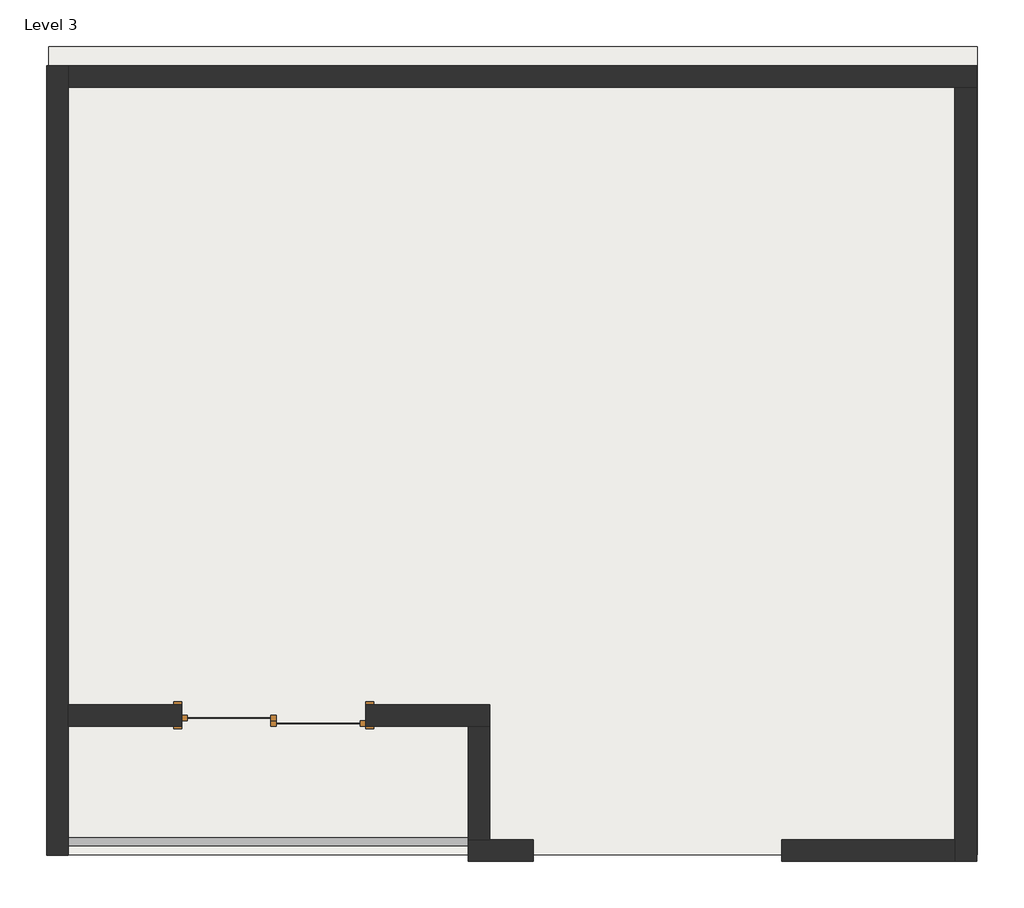
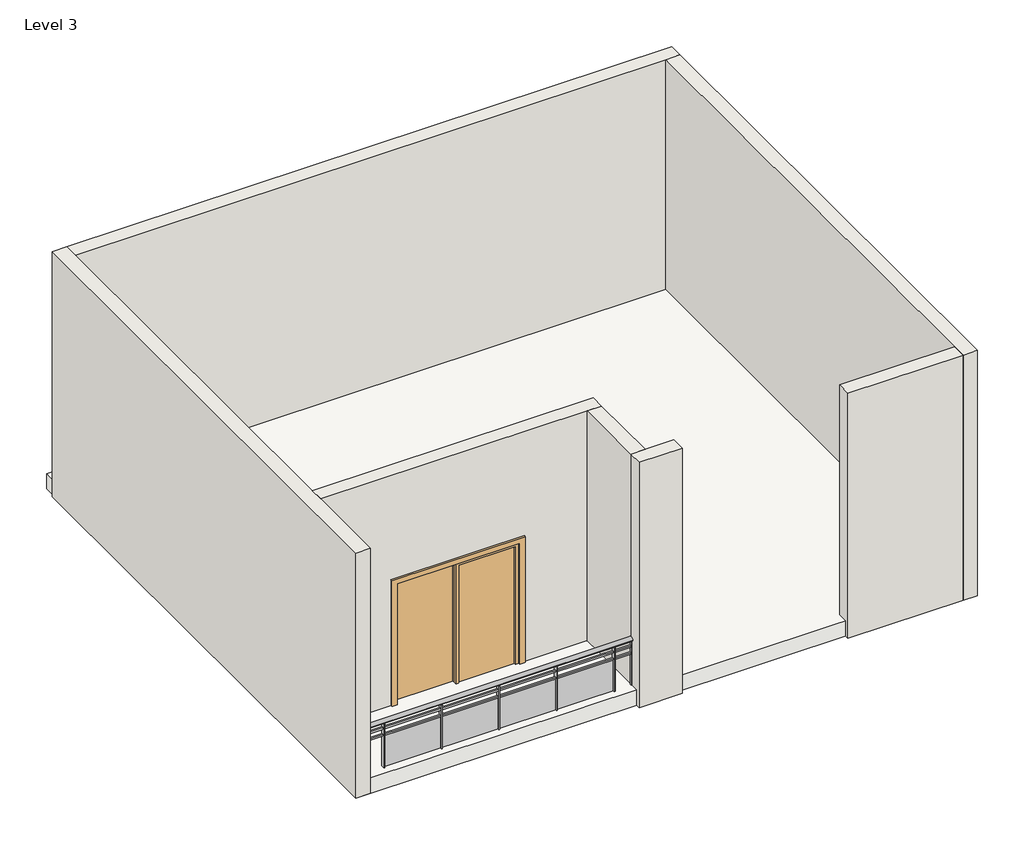
# One storey: 6 walls, 1 door, 1 railing, 1 roof.
"""IFC4 building model written with IfcOpenShell, lengths in millimetres."""

from ifc_helpers import new_model, si_unit, point, frame, origin, place, context, project, spatial, polyline, ellipse_curve, trimmed, outline, extrude, faceted_brep, transform, mapped, element, save
from ifc_brep_helpers import plane_surface, extruded_surface, advanced_brep
from components import door_076b30e0

model = new_model("IFC4")

# Units and contexts
model_context = context("Model", 3, world=origin())
ifc_project = project(units=[si_unit("LENGTHUNIT", "METRE", prefix="MILLI")], contexts=[model_context])

# Site, building, storey
site = spatial("IfcSite", under=ifc_project)
building = spatial("IfcBuilding", under=site)
storey = spatial("IfcBuildingStorey", under=building, Name="Level 3", Elevation=7315.2)

# Door
placement = place(None, origin())
door_shape = door_076b30e0(model_context)
element("IfcDoor", 1, ObjectType="Door-Double-Sliding : 68\" x 80\"", at=placement, inside=storey, context=model_context, shape_type="MappedRepresentation", body=[
    mapped(door_shape, transform((-12322.632922, 6303.7117654, 7315.2), x_axis=(-1.0, 0.0, 0.0), y_axis=(0.0, -1.0, 0.0), z_axis=(0.0, 0.0, 1.0))),
])

# Railing
element("IfcRailing", 2, ObjectType="Glass Panel - Bottom Fill", at=placement, inside=storey, context=model_context, shape_type="SolidModel", body=[
    advanced_brep(
    [(-14253.032922, 5027.3617654, 8229.6), (-14253.032922, 4951.1617654, 8229.6), (-10493.832922, 5027.3617654, 8229.6), (-10493.832922, 4951.1617654, 8229.6)],
    [
        (0, 1, ellipse_curve(frame((-14253.032922, 4989.2617654, 8229.6), z_axis=(-1.0, 0.0, 0.0), x_axis=(0.0, -1.0, 0.0)), 38.1, 28.575)),
        (1, 0, ellipse_curve(frame((-14253.032922, 4989.2617654, 8229.6), z_axis=(-1.0, 0.0, 0.0), x_axis=(0.0, -1.0, 0.0)), 38.1, 28.575)),
        (2, 3, ellipse_curve(frame((-10493.832922, 4989.2617654, 8229.6), z_axis=(1.0, 0.0, 0.0), x_axis=(0.0, -1.0, 0.0)), 38.1, 28.575)),
        (3, 2, ellipse_curve(frame((-10493.832922, 4989.2617654, 8229.6), z_axis=(1.0, 0.0, 0.0), x_axis=(0.0, -1.0, 0.0)), 38.1, 28.575)),
        (0, 2),
        (3, 1),
    ],
    [
        plane_surface(frame((-14253.032922, 4989.2617654, 8229.6), z_axis=(-1.0, 0.0, 0.0), x_axis=(0.0, 1.0, 0.0))),
        plane_surface(frame((-10493.832922, 4989.2617654, 8229.6), z_axis=(1.0, 0.0, 0.0), x_axis=(0.0, 1.0, 0.0))),
        extruded_surface(trimmed(ellipse_curve(frame((-10493.832922, 4989.2617654, 8229.6), z_axis=(-1.0, 0.0, 0.0), x_axis=(0.0, -1.0, 0.0)), 38.1, 28.575), [point((-10493.832922, 5027.3617654, 8229.6))], [point((-10493.832922, 4951.1617654, 8229.6))], True, "CARTESIAN"), (-3759.2000000000007, 0.0, 0.0), 3759.2000000000007),
        extruded_surface(trimmed(ellipse_curve(frame((-10493.832922, 4989.2617654, 8229.6), z_axis=(-1.0, 0.0, 0.0), x_axis=(0.0, -1.0, 0.0)), 38.1, 28.575), [point((-10493.832922, 4951.1617654, 8229.6))], [point((-10493.832922, 5027.3617654, 8229.6))], True, "CARTESIAN"), (-3759.2000000000007, 0.0, 0.0), 3759.2000000000007),
    ],
    [
        (0, [[1, 2]]),
        (1, [[3, 4]]),
        (2, [[-1, 5, -4, 6]]),
        (3, [[-2, -6, -3, -5]]),
    ],
),
    extrude(outline(polyline([(-14253.032922, 4976.5617654), (-14253.032922, 5001.9617654), (-10493.832922, 5001.9617654), (-10493.832922, 4976.5617654), (-14253.032922, 4976.5617654)])), frame((0.0, 0.0, 8115.3), z_axis=(0.0, 0.0, 1.0), x_axis=(1.0, 0.0, 0.0)), (0.0, 0.0, 1.0), 25.4),
    extrude(outline(polyline([(-14253.032922, 4976.5617654), (-14253.032922, 5001.9617654), (-10493.832922, 5001.9617654), (-10493.832922, 4976.5617654), (-14253.032922, 4976.5617654)])), frame((0.0, 0.0, 8013.7), z_axis=(0.0, 0.0, 1.0), x_axis=(1.0, 0.0, 0.0)), (0.0, 0.0, 1.0), 25.4),
    extrude(outline(polyline([(-10754.182922, 4963.8617654), (-10754.182922, 5014.6617654), (-10741.482922, 5014.6617654), (-10741.482922, 4963.8617654), (-10754.182922, 4963.8617654)])), frame((0.0, 0.0, 7315.2), z_axis=(0.0, 0.0, 1.0), x_axis=(1.0, 0.0, 0.0)), (0.0, 0.0, 1.0), 885.6788223),
    extrude(outline(polyline([(-11560.632922, 4995.7969224), (-10747.832922, 4995.7969224), (-10747.832922, 4989.4469224), (-11560.632922, 4989.4469224), (-11560.632922, 4995.7969224)])), frame((0.0, 0.0, 7416.8), z_axis=(0.0, 0.0, 1.0), x_axis=(1.0, 0.0, 0.0)), (0.0, 0.0, 1.0), 596.9),
    extrude(outline(polyline([(-11566.982922, 4963.8617654), (-11566.982922, 5014.6617654), (-11554.282922, 5014.6617654), (-11554.282922, 4963.8617654), (-11566.982922, 4963.8617654)])), frame((0.0, 0.0, 7315.2), z_axis=(0.0, 0.0, 1.0), x_axis=(1.0, 0.0, 0.0)), (0.0, 0.0, 1.0), 885.6788223),
    extrude(outline(polyline([(-12373.432922, 4995.7969224), (-11560.632922, 4995.7969224), (-11560.632922, 4989.4469224), (-12373.432922, 4989.4469224), (-12373.432922, 4995.7969224)])), frame((0.0, 0.0, 7416.8), z_axis=(0.0, 0.0, 1.0), x_axis=(1.0, 0.0, 0.0)), (0.0, 0.0, 1.0), 596.9),
    extrude(outline(polyline([(-12379.782922, 4963.8617654), (-12379.782922, 5014.6617654), (-12367.082922, 5014.6617654), (-12367.082922, 4963.8617654), (-12379.782922, 4963.8617654)])), frame((0.0, 0.0, 7315.2), z_axis=(0.0, 0.0, 1.0), x_axis=(1.0, 0.0, 0.0)), (0.0, 0.0, 1.0), 885.6788223),
    extrude(outline(polyline([(-13186.232922, 4995.7969224), (-12373.432922, 4995.7969224), (-12373.432922, 4989.4469224), (-13186.232922, 4989.4469224), (-13186.232922, 4995.7969224)])), frame((0.0, 0.0, 7416.8), z_axis=(0.0, 0.0, 1.0), x_axis=(1.0, 0.0, 0.0)), (0.0, 0.0, 1.0), 596.9),
    extrude(outline(polyline([(-13192.582922, 4963.8617654), (-13192.582922, 5014.6617654), (-13179.882922, 5014.6617654), (-13179.882922, 4963.8617654), (-13192.582922, 4963.8617654)])), frame((0.0, 0.0, 7315.2), z_axis=(0.0, 0.0, 1.0), x_axis=(1.0, 0.0, 0.0)), (0.0, 0.0, 1.0), 885.6788223),
    extrude(outline(polyline([(-13999.032922, 4995.7969224), (-13186.232922, 4995.7969224), (-13186.232922, 4989.4469224), (-13999.032922, 4989.4469224), (-13999.032922, 4995.7969224)])), frame((0.0, 0.0, 7416.8), z_axis=(0.0, 0.0, 1.0), x_axis=(1.0, 0.0, 0.0)), (0.0, 0.0, 1.0), 596.9),
    extrude(outline(polyline([(-14005.382922, 4963.8617654), (-14005.382922, 5014.6617654), (-13992.682922, 5014.6617654), (-13992.682922, 4963.8617654), (-14005.382922, 4963.8617654)])), frame((0.0, 0.0, 7315.2), z_axis=(0.0, 0.0, 1.0), x_axis=(1.0, 0.0, 0.0)), (0.0, 0.0, 1.0), 885.6788223),
    extrude(outline(polyline([(-10506.532922, 4979.7367654), (-10506.532922, 4998.7867654), (-10487.482922, 4998.7867654), (-10487.482922, 4979.7367654), (-10506.532922, 4979.7367654)])), frame((0.0, 0.0, 7315.2), z_axis=(0.0, 0.0, 1.0), x_axis=(1.0, 0.0, 0.0)), (0.0, 0.0, 1.0), 885.6788223),
    extrude(outline(polyline([(-14259.382922, 4979.7367654), (-14259.382922, 4998.7867654), (-14240.332922, 4998.7867654), (-14240.332922, 4979.7367654), (-14259.382922, 4979.7367654)])), frame((0.0, 0.0, 7315.2), z_axis=(0.0, 0.0, 1.0), x_axis=(1.0, 0.0, 0.0)), (0.0, 0.0, 1.0), 885.6788223),
])

# Roof
element("IfcRoof", 3, ObjectType="Generic - 9\"", at=placement, inside=storey, context=model_context, shape_type="SweptSolid", body=[
    extrude(outline(polyline([(-14435.2593035, 12460.3935836), (-5710.3593035, 12460.3935836), (-5710.3593035, 4865.7935836), (-10301.4093035, 4865.7935836), (-14435.2593035, 4865.7935836), (-14435.2593035, 12460.3935836)])), frame((0.0, 0.0, 7315.2), z_axis=(0.0, 0.0, 1.0), x_axis=(1.0, 0.0, 0.0)), (0.0, 0.0, 1.0), 228.6),
])

# Walls
element("IfcWall", 4, ObjectType="Generic - 8\"", at=placement, inside=storey, context=model_context, shape_type="Brep", body=[
    faceted_brep([(-14253.032922, 4862.2617654, 7315.2), (-14253.032922, 6075.1117654, 7315.2), (-14253.032922, 6278.3117654, 7315.2), (-14253.032922, 12075.8617654, 7315.2), (-14253.032922, 12279.0617654, 7315.2), (-14253.032922, 12279.0617654, 10972.8), (-14253.032922, 12075.8617654, 10972.8), (-14253.032922, 6278.3117654, 10972.8), (-14253.032922, 6075.1117654, 10972.8), (-14253.032922, 4862.2617654, 10972.8), (-14456.232922, 4862.2617654, 7315.2), (-14456.232922, 4862.2617654, 10972.8), (-14456.232922, 12279.0617654, 10972.8), (-14456.232922, 12279.0617654, 7315.2), (-14456.232922, 12075.8617654, 7315.2), (-14456.232922, 6075.1117654, 7315.2)], [[[0, 1, 2, 3, 4, 5, 6, 7, 8, 9]], [[10, 11, 12, 13, 14, 15]], [[4, 3, 2, 1, 0, 10, 15, 14, 13]], [[9, 8, 7, 6, 5, 12, 11]], [[0, 9, 11, 10]], [[5, 4, 13, 12]]]),
])
element("IfcWall", 5, ObjectType="Generic - 8\"", at=placement, inside=storey, context=model_context, shape_type="Brep", body=[
    faceted_brep([(-14253.032922, 12075.8617654, 7315.2), (-5921.832922, 12075.8617654, 7315.2), (-5718.632922, 12075.8617654, 7315.2), (-5718.632922, 12075.8617654, 10972.8), (-5921.832922, 12075.8617654, 10972.8), (-14253.032922, 12075.8617654, 10972.8), (-14253.032922, 12279.0617654, 7315.2), (-14253.032922, 12279.0617654, 10972.8), (-5718.632922, 12279.0617654, 10972.8), (-5718.632922, 12279.0617654, 7315.2)], [[[0, 1, 2, 3, 4, 5]], [[6, 7, 8, 9]], [[2, 1, 0, 6, 9]], [[5, 4, 3, 8, 7]], [[3, 2, 9, 8]], [[0, 5, 7, 6]]]),
])
element("IfcWall", 6, ObjectType="Generic - 8\"", at=placement, inside=storey, context=model_context, shape_type="Brep", body=[
    faceted_brep([(-5921.832922, 12075.8617654, 7315.2), (-5921.832922, 5008.3117654, 7315.2), (-5921.832922, 4805.1117654, 7315.2), (-5921.832922, 4805.1117654, 10972.8), (-5921.832922, 5008.3117654, 10972.8), (-5921.832922, 12075.8617654, 10972.8), (-5718.632922, 12075.8617654, 7315.2), (-5718.632922, 12075.8617654, 10972.8), (-5718.632922, 4805.1117654, 10972.8), (-5718.632922, 4805.1117654, 7315.2)], [[[0, 1, 2, 3, 4, 5]], [[6, 7, 8, 9]], [[2, 1, 0, 6, 9]], [[5, 4, 3, 8, 7]], [[0, 5, 7, 6]], [[3, 2, 9, 8]]]),
])
element("IfcWall", 7, ObjectType="Generic - 8\"", at=placement, inside=storey, context=model_context, shape_type="Brep", body=[
    faceted_brep([(-5921.832922, 5008.3117654, 7315.2), (-7547.432922, 5008.3117654, 7315.2), (-7547.432922, 5008.3117654, 10972.8), (-5921.832922, 5008.3117654, 10972.8), (-5921.832922, 4805.1117654, 7315.2), (-5921.832922, 4805.1117654, 10972.8), (-7547.432922, 4805.1117654, 10972.8), (-7547.432922, 4805.1117654, 7315.2)], [[[0, 1, 2, 3]], [[4, 5, 6, 7]], [[0, 3, 5, 4]], [[1, 0, 4, 7]], [[2, 1, 7, 6]], [[3, 2, 6, 5]]]),
    faceted_brep([(-10493.832922, 5008.3117654, 10972.8), (-10290.632922, 5008.3117654, 10972.8), (-9884.232922, 5008.3117654, 10972.8), (-9884.232922, 5008.3117654, 7315.2), (-10290.632922, 5008.3117654, 7315.2), (-10493.832922, 5008.3117654, 7315.2), (-10493.832922, 4805.1117654, 10972.8), (-10493.832922, 4805.1117654, 7315.2), (-9884.232922, 4805.1117654, 7315.2), (-9884.232922, 4805.1117654, 10972.8)], [[[0, 1, 2, 3, 4, 5]], [[6, 7, 8, 9]], [[0, 5, 7, 6]], [[2, 1, 0, 6, 9]], [[3, 2, 9, 8]], [[5, 4, 3, 8, 7]]]),
])
element("IfcWall", 8, ObjectType="Generic - 8\"", at=placement, inside=storey, context=model_context, shape_type="Brep", body=[
    faceted_brep([(-14253.032922, 6075.1117654, 7315.2), (-13186.232922, 6075.1117654, 7315.2), (-13186.232922, 6075.1117654, 9347.2), (-11459.032922, 6075.1117654, 9347.2), (-11459.032922, 6075.1117654, 7315.2), (-10493.832922, 6075.1117654, 7315.2), (-10290.632922, 6075.1117654, 7315.2), (-10290.632922, 6075.1117654, 10972.8), (-10493.832922, 6075.1117654, 10972.8), (-14253.032922, 6075.1117654, 10972.8), (-13186.232922, 6278.3117654, 9347.2), (-13186.232922, 6278.3117654, 7315.2), (-14253.032922, 6278.3117654, 7315.2), (-14253.032922, 6278.3117654, 10972.8), (-10290.632922, 6278.3117654, 10972.8), (-10290.632922, 6278.3117654, 7315.2), (-11459.032922, 6278.3117654, 7315.2), (-11459.032922, 6278.3117654, 9347.2)], [[[0, 1, 2, 3, 4, 5, 6, 7, 8, 9]], [[10, 11, 12, 13, 14, 15, 16, 17]], [[12, 11, 1, 0]], [[16, 15, 6, 5, 4]], [[9, 8, 7, 14, 13]], [[0, 9, 13, 12]], [[7, 6, 15, 14]], [[4, 3, 17, 16]], [[2, 1, 11, 10]], [[3, 2, 10, 17]]]),
])
element("IfcWall", 9, ObjectType="Generic - 8\"", at=placement, inside=storey, context=model_context, shape_type="SweptSolid", body=[
    extrude(outline(polyline([(-10493.832922, 5008.3117654), (-10493.832922, 6075.1117654), (-10290.632922, 6075.1117654), (-10290.632922, 5008.3117654), (-10493.832922, 5008.3117654)])), frame((0.0, 0.0, 7315.2), z_axis=(0.0, 0.0, 1.0), x_axis=(1.0, 0.0, 0.0)), (0.0, 0.0, 1.0), 3657.6),
])

save(model, "model.ifc")

# Revit data of these elements
# Type "Door-Double-Sliding : 68\" x 80\""
#   Type Mark = "8"
#   Construction Type Id = "opn-d45"
#   Assembly Code = "C1020"
#   Analytic Construction = "Wood frame, double glass door "
#   Thickness = 0' - 2"
#   Thermal Resistance (R) = 1.8150 (h·ft²·°F)/BTU
#   Heat Transfer Coefficient (U) = 0.5510 BTU/(h·ft²·°F)
#   Height = 6' - 8"
#   Rail Width = 0' - 2"
#   Stiles = 0' - 2"
#   Trim Projection Ext = 0' - 1"
#   Trim Projection Int = 0' - 1"
#   Trim Width = 0' - 3"
#   Width = 5' - 8"
#   Define Thermal Properties by = 1
#   Glazing = Glass
#   Panel Material = Wood - Birch - Solid Stained Light Low Gloss
#   Trim Material = Paint - Sienna
#   Visual Light Transmittance = 0
#   Solar Heat Gain Coefficient = 0
#   Function = (empty or 0)
#   Wall Closure = (empty or 0)
# Type "Glass Panel - Bottom Fill"
#   Assembly Code = "C2010400"
#   built-in parameter 1008612 = 0.0416667 (stored number, unit not read)
#   built-in parameter 1008611 = 0.0416667 (stored number, unit not read)
#   built-in parameter 1008609 = 0.333333 (stored number, unit not read)
#   built-in parameter 1008604 = 0.166667 (stored number, unit not read)
#   built-in parameter 1008603 = 0.166667 (stored number, unit not read)
#   Railing Height = 3' - 0"
#   built-in parameter 1008630 = 2
#   built-in parameter 1008610 = 2
#   built-in parameter 1008618 = Baluster - Square : 3/4"
# Type "Generic - 9\""
#   Assembly Code = "B1020"
#   Layers, outside or top first: 0' - 9" no material (function 1)
# Type "Generic - 8\""
#   Assembly Code = "B2010"
#   Layers, outside or top first: 0' - 8" no material (function 1)
# Element 1 (IfcDoor, "Door-Double-Sliding : 68\" x 80\"")
#   Phase Created = New Construction
#   Materials on its faces: "Paint - Sienna", "Wood - Birch - Solid Stained Light Low Gloss", "Glass"
# Element 2 (IfcRailing, "Glass Panel - Bottom Fill")
#   Phase Created = New Construction
#   Materials on its faces: "Glass"
# Element 3 (IfcRoof, "Generic - 9\"")
#   built-in parameter 1001705 = 24.75 (stored number, unit not read)
#   built-in parameter 1001710 = 33615
#   Phase Created = New Construction
#   Materials on its faces: "Default Roof"
# Elements 4, 5, 6, 7, 8, 9 (IfcWall, "Generic - 8\"")
#   Top Offset = 0' - 0"
#   Base Offset = 0' - 0"
#   Unconnected Height = 12' - 0"
#   wall height = 12' - 0"
#   Phase Created = New Construction
#   Base Constraint = Level 3
#   Materials on its faces: "Default Wall"
# Materials
#   "Glass": class "Glass", colour RGB 0 128 192, transparency 0.75, Description = "Soda Lime Glass", Cost = 0
#   "Wood - Birch - Solid Stained Light Low Gloss": class "Wood", colour RGB 210 159 95, transparency 0, Cost = 0
#   "Paint - Sienna": colour RGB 118 70 51, transparency 0, Cost = 0
#   "Default Roof": colour RGB 88 101 114, transparency 0
#   "Default Wall": colour RGB 128 128 128, transparency 0
